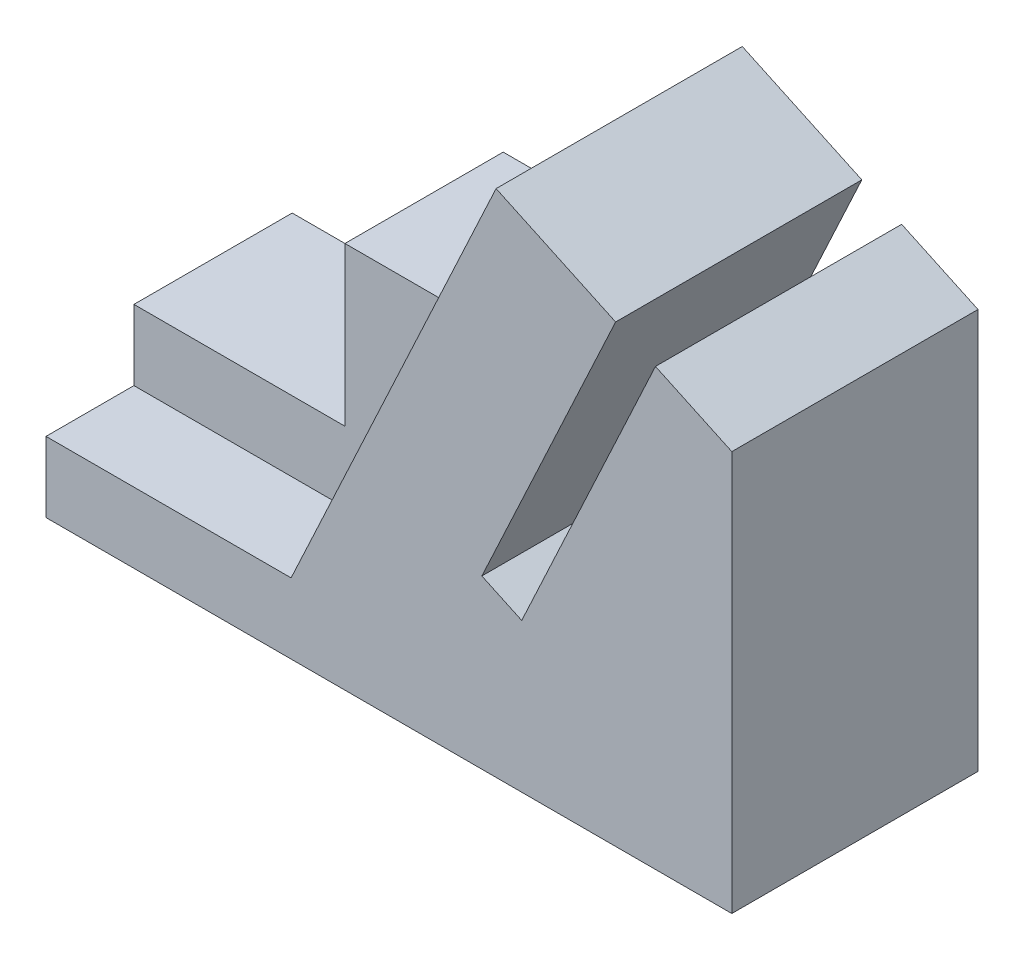
ISO-10303-21;
HEADER;
FILE_DESCRIPTION(('STEP AP214'),'2;1');
FILE_NAME('part.step','',(''),(''),'','','');
FILE_SCHEMA(('AUTOMOTIVE_DESIGN { 1 0 10303 214 1 1 1 1 }'));
ENDSEC;
DATA;
#1=APPLICATION_CONTEXT('core data for automotive mechanical design processes');
#2=APPLICATION_PROTOCOL_DEFINITION('international standard','automotive_design',2000,#1);
#3=PRODUCT_CONTEXT('',#1,'mechanical');
#4=PRODUCT('Part','Part','',(#3));
#5=PRODUCT_RELATED_PRODUCT_CATEGORY('part','',(#4));
#6=PRODUCT_DEFINITION_FORMATION('','',#4);
#7=PRODUCT_DEFINITION_CONTEXT('part definition',#1,'design');
#8=PRODUCT_DEFINITION('design','',#6,#7);
#9=PRODUCT_DEFINITION_SHAPE('','',#8);
#10=(LENGTH_UNIT() NAMED_UNIT(*) SI_UNIT(.MILLI.,.METRE.));
#11=(NAMED_UNIT(*) PLANE_ANGLE_UNIT() SI_UNIT($,.RADIAN.));
#12=(NAMED_UNIT(*) SI_UNIT($,.STERADIAN.) SOLID_ANGLE_UNIT());
#13=UNCERTAINTY_MEASURE_WITH_UNIT(LENGTH_MEASURE(1.E-05),#10,'distance_accuracy_value','');
#14=(GEOMETRIC_REPRESENTATION_CONTEXT(3) GLOBAL_UNCERTAINTY_ASSIGNED_CONTEXT((#13)) GLOBAL_UNIT_ASSIGNED_CONTEXT((#10,
#11,#12)) REPRESENTATION_CONTEXT('',''));
#15=CARTESIAN_POINT('',(0.,0.,0.));
#16=DIRECTION('',(0.,0.,1.));
#17=DIRECTION('',(1.,0.,0.));
#18=AXIS2_PLACEMENT_3D('',#15,#16,#17);
#19=CARTESIAN_POINT('',(0.,0.,3.99999999999999));
#20=DIRECTION('',(0.,0.,-1.));
#21=DIRECTION('',(-1.,0.,0.));
#22=AXIS2_PLACEMENT_3D('',#19,#20,#21);
#23=PLANE('',#22);
#24=DIRECTION('',(-0.422618261740697,-0.906307787036651,0.));
#25=VECTOR('',#24,1.);
#26=CARTESIAN_POINT('',(-12.2013617281793,5.68958841376926,3.99999999999999));
#27=LINE('',#26,#25);
#28=CARTESIAN_POINT('',(1.00000000000001,34.,3.99999999999999));
#29=VERTEX_POINT('',#28);
#30=CARTESIAN_POINT('',(-11.1239991120298,8.,3.99999999999999));
#31=VERTEX_POINT('',#30);
#32=EDGE_CURVE('E11',#29,#31,#27,.T.);
#33=ORIENTED_EDGE('',*,*,#32,.F.);
#34=DIRECTION('',(1.,0.,0.));
#35=VECTOR('',#34,1.);
#36=CARTESIAN_POINT('',(-15.,34.,3.99999999999999));
#37=LINE('',#36,#35);
#38=CARTESIAN_POINT('',(-15.,34.,3.99999999999999));
#39=VERTEX_POINT('',#38);
#40=EDGE_CURVE('E203',#39,#29,#37,.T.);
#41=ORIENTED_EDGE('',*,*,#40,.F.);
#42=DIRECTION('',(0.,1.,0.));
#43=VECTOR('',#42,1.);
#44=CARTESIAN_POINT('',(-15.,16.,3.99999999999999));
#45=LINE('',#44,#43);
#46=CARTESIAN_POINT('',(-15.,16.,3.99999999999999));
#47=VERTEX_POINT('',#46);
#48=EDGE_CURVE('E196',#47,#39,#45,.T.);
#49=ORIENTED_EDGE('',*,*,#48,.F.);
#50=DIRECTION('',(1.,0.,0.));
#51=VECTOR('',#50,1.);
#52=CARTESIAN_POINT('',(-39.,16.,3.99999999999999));
#53=LINE('',#52,#51);
#54=CARTESIAN_POINT('',(-39.,16.,3.99999999999999));
#55=VERTEX_POINT('',#54);
#56=EDGE_CURVE('E194',#55,#47,#53,.T.);
#57=ORIENTED_EDGE('',*,*,#56,.F.);
#58=DIRECTION('',(0.,1.,0.));
#59=VECTOR('',#58,1.);
#60=CARTESIAN_POINT('',(-39.,8.,3.99999999999999));
#61=LINE('',#60,#59);
#62=CARTESIAN_POINT('',(-39.,8.,3.99999999999999));
#63=VERTEX_POINT('',#62);
#64=EDGE_CURVE('E191',#63,#55,#61,.T.);
#65=ORIENTED_EDGE('',*,*,#64,.F.);
#66=DIRECTION('',(-1.,0.,0.));
#67=VECTOR('',#66,1.);
#68=CARTESIAN_POINT('',(1.00000000000001,8.,3.99999999999999));
#69=LINE('',#68,#67);
#70=EDGE_CURVE('E56',#31,#63,#69,.T.);
#71=ORIENTED_EDGE('',*,*,#70,.F.);
#72=EDGE_LOOP('',(#33,#41,#49,#57,#65,#71));
#73=FACE_BOUND('',#72,.T.);
#74=ADVANCED_FACE('F39',(#73),#23,.F.);
#75=CARTESIAN_POINT('',(39.,8.,-14.));
#76=DIRECTION('',(-1.,0.,0.));
#77=DIRECTION('',(0.,0.,1.));
#78=AXIS2_PLACEMENT_3D('',#75,#76,#77);
#79=PLANE('',#78);
#80=DIRECTION('',(0.,0.,-1.));
#81=VECTOR('',#80,1.);
#82=CARTESIAN_POINT('',(39.,0.,-14.));
#83=LINE('',#82,#81);
#84=CARTESIAN_POINT('',(39.,0.,14.));
#85=VERTEX_POINT('',#84);
#86=CARTESIAN_POINT('',(39.,0.,-14.));
#87=VERTEX_POINT('',#86);
#88=EDGE_CURVE('E214',#85,#87,#83,.T.);
#89=ORIENTED_EDGE('',*,*,#88,.T.);
#90=DIRECTION('',(0.,-1.,0.));
#91=VECTOR('',#90,1.);
#92=CARTESIAN_POINT('',(39.,8.,-14.));
#93=LINE('',#92,#91);
#94=CARTESIAN_POINT('',(39.,45.4989369594061,-14.));
#95=VERTEX_POINT('',#94);
#96=EDGE_CURVE('E50',#95,#87,#93,.T.);
#97=ORIENTED_EDGE('',*,*,#96,.F.);
#98=DIRECTION('',(0.,0.,1.));
#99=VECTOR('',#98,1.);
#100=CARTESIAN_POINT('',(39.,45.4989369594061,-84.7984130258777));
#101=LINE('',#100,#99);
#102=CARTESIAN_POINT('',(39.,45.4989369594061,14.));
#103=VERTEX_POINT('',#102);
#104=EDGE_CURVE('E179',#95,#103,#101,.T.);
#105=ORIENTED_EDGE('',*,*,#104,.T.);
#106=DIRECTION('',(0.,-1.,0.));
#107=VECTOR('',#106,1.);
#108=CARTESIAN_POINT('',(39.,8.,14.));
#109=LINE('',#108,#107);
#110=EDGE_CURVE('E229',#103,#85,#109,.T.);
#111=ORIENTED_EDGE('',*,*,#110,.T.);
#112=EDGE_LOOP('',(#89,#97,#105,#111));
#113=FACE_BOUND('',#112,.T.);
#114=ADVANCED_FACE('F41',(#113),#79,.F.);
#115=CARTESIAN_POINT('',(-39.,8.,-14.));
#116=DIRECTION('',(0.,0.,1.));
#117=DIRECTION('',(1.,0.,0.));
#118=AXIS2_PLACEMENT_3D('',#115,#116,#117);
#119=PLANE('',#118);
#120=DIRECTION('',(1.,0.,0.));
#121=VECTOR('',#120,1.);
#122=CARTESIAN_POINT('',(-15.,34.,-14.));
#123=LINE('',#122,#121);
#124=CARTESIAN_POINT('',(-15.,34.,-14.));
#125=VERTEX_POINT('',#124);
#126=CARTESIAN_POINT('',(1.00000000000001,34.,-14.));
#127=VERTEX_POINT('',#126);
#128=EDGE_CURVE('E195',#125,#127,#123,.T.);
#129=ORIENTED_EDGE('',*,*,#128,.T.);
#130=DIRECTION('',(-0.422618261740697,-0.906307787036651,0.));
#131=VECTOR('',#130,1.);
#132=CARTESIAN_POINT('',(-11.1239991120298,8.,-14.));
#133=LINE('',#132,#131);
#134=CARTESIAN_POINT('',(12.1913837957199,58.,-14.));
#135=VERTEX_POINT('',#134);
#136=EDGE_CURVE('E167',#135,#127,#133,.T.);
#137=ORIENTED_EDGE('',*,*,#136,.F.);
#138=DIRECTION('',(-0.906307787036651,0.422618261740696,0.));
#139=VECTOR('',#138,1.);
#140=CARTESIAN_POINT('',(12.1913837957199,58.,-14.));
#141=LINE('',#140,#139);
#142=CARTESIAN_POINT('',(25.7860006012697,51.6607260738895,-14.));
#143=VERTEX_POINT('',#142);
#144=EDGE_CURVE('E148',#143,#135,#141,.T.);
#145=ORIENTED_EDGE('',*,*,#144,.F.);
#146=DIRECTION('',(0.422618261740697,0.906307787036651,0.));
#147=VECTOR('',#146,1.);
#148=CARTESIAN_POINT('',(25.7860006012697,51.6607260738895,-14.));
#149=LINE('',#148,#147);
#150=CARTESIAN_POINT('',(10.5717431786046,19.0336457405701,-14.));
#151=VERTEX_POINT('',#150);
#152=EDGE_CURVE('E273',#151,#143,#149,.T.);
#153=ORIENTED_EDGE('',*,*,#152,.F.);
#154=DIRECTION('',(-0.906307787036651,0.422618261740696,0.));
#155=VECTOR('',#154,1.);
#156=CARTESIAN_POINT('',(10.5717431786046,19.0336457405701,-14.));
#157=LINE('',#156,#155);
#158=CARTESIAN_POINT('',(15.1032821137878,16.9205544318666,-14.));
#159=VERTEX_POINT('',#158);
#160=EDGE_CURVE('E269',#159,#151,#157,.T.);
#161=ORIENTED_EDGE('',*,*,#160,.F.);
#162=DIRECTION('',(-0.422618261740696,-0.906307787036652,0.));
#163=VECTOR('',#162,1.);
#164=CARTESIAN_POINT('',(15.1032821137878,16.9205544318666,-14.));
#165=LINE('',#164,#163);
#166=CARTESIAN_POINT('',(30.3175395364529,49.5476347651861,-14.));
#167=VERTEX_POINT('',#166);
#168=EDGE_CURVE('E277',#167,#159,#165,.T.);
#169=ORIENTED_EDGE('',*,*,#168,.F.);
#170=DIRECTION('',(-0.906307787036652,0.422618261740696,0.));
#171=VECTOR('',#170,1.);
#172=CARTESIAN_POINT('',(30.3175395364529,49.5476347651861,-14.));
#173=LINE('',#172,#171);
#174=EDGE_CURVE('E147',#95,#167,#173,.T.);
#175=ORIENTED_EDGE('',*,*,#174,.F.);
#176=ORIENTED_EDGE('',*,*,#96,.T.);
#177=DIRECTION('',(-1.,0.,0.));
#178=VECTOR('',#177,1.);
#179=CARTESIAN_POINT('',(-39.,0.,-14.));
#180=LINE('',#179,#178);
#181=CARTESIAN_POINT('',(-39.,0.,-14.));
#182=VERTEX_POINT('',#181);
#183=EDGE_CURVE('E228',#87,#182,#180,.T.);
#184=ORIENTED_EDGE('',*,*,#183,.T.);
#185=DIRECTION('',(0.,-1.,0.));
#186=VECTOR('',#185,1.);
#187=CARTESIAN_POINT('',(-39.,8.,-14.));
#188=LINE('',#187,#186);
#189=CARTESIAN_POINT('',(-39.,16.,-14.));
#190=VERTEX_POINT('',#189);
#191=EDGE_CURVE('E239',#190,#182,#188,.T.);
#192=ORIENTED_EDGE('',*,*,#191,.F.);
#193=DIRECTION('',(1.,0.,0.));
#194=VECTOR('',#193,1.);
#195=CARTESIAN_POINT('',(-39.,16.,-14.));
#196=LINE('',#195,#194);
#197=CARTESIAN_POINT('',(-15.,16.,-14.));
#198=VERTEX_POINT('',#197);
#199=EDGE_CURVE('E202',#190,#198,#196,.T.);
#200=ORIENTED_EDGE('',*,*,#199,.T.);
#201=DIRECTION('',(0.,1.,0.));
#202=VECTOR('',#201,1.);
#203=CARTESIAN_POINT('',(-15.,16.,-14.));
#204=LINE('',#203,#202);
#205=EDGE_CURVE('E208',#198,#125,#204,.T.);
#206=ORIENTED_EDGE('',*,*,#205,.T.);
#207=EDGE_LOOP('',(#129,#137,#145,#153,#161,#169,#175,#176,#184,#192,#200,#206));
#208=FACE_BOUND('',#207,.T.);
#209=ADVANCED_FACE('F243',(#208),#119,.F.);
#210=CARTESIAN_POINT('',(-39.,8.,-14.));
#211=DIRECTION('',(1.,0.,0.));
#212=DIRECTION('',(0.,0.,-1.));
#213=AXIS2_PLACEMENT_3D('',#210,#211,#212);
#214=PLANE('',#213);
#215=DIRECTION('',(0.,0.,1.));
#216=VECTOR('',#215,1.);
#217=CARTESIAN_POINT('',(-39.,0.,-14.));
#218=LINE('',#217,#216);
#219=CARTESIAN_POINT('',(-39.,0.,14.));
#220=VERTEX_POINT('',#219);
#221=EDGE_CURVE('E231',#182,#220,#218,.T.);
#222=ORIENTED_EDGE('',*,*,#221,.T.);
#223=DIRECTION('',(0.,-1.,0.));
#224=VECTOR('',#223,1.);
#225=CARTESIAN_POINT('',(-39.,8.,14.));
#226=LINE('',#225,#224);
#227=CARTESIAN_POINT('',(-39.,8.,14.));
#228=VERTEX_POINT('',#227);
#229=EDGE_CURVE('E237',#228,#220,#226,.T.);
#230=ORIENTED_EDGE('',*,*,#229,.F.);
#231=DIRECTION('',(0.,0.,1.));
#232=VECTOR('',#231,1.);
#233=CARTESIAN_POINT('',(-39.,8.,-14.));
#234=LINE('',#233,#232);
#235=EDGE_CURVE('E225',#63,#228,#234,.T.);
#236=ORIENTED_EDGE('',*,*,#235,.F.);
#237=ORIENTED_EDGE('',*,*,#64,.T.);
#238=DIRECTION('',(0.,0.,-1.));
#239=VECTOR('',#238,1.);
#240=CARTESIAN_POINT('',(-39.,16.,3.99999999999999));
#241=LINE('',#240,#239);
#242=EDGE_CURVE('E204',#55,#190,#241,.T.);
#243=ORIENTED_EDGE('',*,*,#242,.T.);
#244=ORIENTED_EDGE('',*,*,#191,.T.);
#245=EDGE_LOOP('',(#222,#230,#236,#237,#243,#244));
#246=FACE_BOUND('',#245,.T.);
#247=ADVANCED_FACE('F254',(#246),#214,.F.);
#248=CARTESIAN_POINT('',(-39.,8.,14.));
#249=DIRECTION('',(0.,0.,-1.));
#250=DIRECTION('',(-1.,0.,0.));
#251=AXIS2_PLACEMENT_3D('',#248,#249,#250);
#252=PLANE('',#251);
#253=DIRECTION('',(1.,0.,0.));
#254=VECTOR('',#253,1.);
#255=CARTESIAN_POINT('',(-39.,0.,14.));
#256=LINE('',#255,#254);
#257=EDGE_CURVE('E221',#220,#85,#256,.T.);
#258=ORIENTED_EDGE('',*,*,#257,.T.);
#259=ORIENTED_EDGE('',*,*,#110,.F.);
#260=DIRECTION('',(0.906307787036651,-0.422618261740696,0.));
#261=VECTOR('',#260,1.);
#262=CARTESIAN_POINT('',(30.3175395364529,49.5476347651861,14.));
#263=LINE('',#262,#261);
#264=CARTESIAN_POINT('',(30.3175395364529,49.5476347651861,14.));
#265=VERTEX_POINT('',#264);
#266=EDGE_CURVE('E176',#265,#103,#263,.T.);
#267=ORIENTED_EDGE('',*,*,#266,.F.);
#268=DIRECTION('',(0.422618261740696,0.906307787036651,0.));
#269=VECTOR('',#268,1.);
#270=CARTESIAN_POINT('',(15.1032821137878,16.9205544318666,14.));
#271=LINE('',#270,#269);
#272=CARTESIAN_POINT('',(15.1032821137878,16.9205544318666,14.));
#273=VERTEX_POINT('',#272);
#274=EDGE_CURVE('E175',#273,#265,#271,.T.);
#275=ORIENTED_EDGE('',*,*,#274,.F.);
#276=DIRECTION('',(0.906307787036652,-0.422618261740696,0.));
#277=VECTOR('',#276,1.);
#278=CARTESIAN_POINT('',(10.5717431786046,19.0336457405701,14.));
#279=LINE('',#278,#277);
#280=CARTESIAN_POINT('',(10.5717431786046,19.0336457405701,14.));
#281=VERTEX_POINT('',#280);
#282=EDGE_CURVE('E168',#281,#273,#279,.T.);
#283=ORIENTED_EDGE('',*,*,#282,.F.);
#284=DIRECTION('',(-0.422618261740696,-0.906307787036651,0.));
#285=VECTOR('',#284,1.);
#286=CARTESIAN_POINT('',(25.7860006012697,51.6607260738895,14.));
#287=LINE('',#286,#285);
#288=CARTESIAN_POINT('',(25.7860006012697,51.6607260738895,14.));
#289=VERTEX_POINT('',#288);
#290=EDGE_CURVE('E157',#289,#281,#287,.T.);
#291=ORIENTED_EDGE('',*,*,#290,.F.);
#292=DIRECTION('',(0.906307787036651,-0.422618261740696,0.));
#293=VECTOR('',#292,1.);
#294=CARTESIAN_POINT('',(12.1913837957199,58.,14.));
#295=LINE('',#294,#293);
#296=CARTESIAN_POINT('',(12.1913837957199,58.,14.));
#297=VERTEX_POINT('',#296);
#298=EDGE_CURVE('E145',#297,#289,#295,.T.);
#299=ORIENTED_EDGE('',*,*,#298,.F.);
#300=DIRECTION('',(0.422618261740697,0.906307787036651,0.));
#301=VECTOR('',#300,1.);
#302=CARTESIAN_POINT('',(-11.1239991120298,8.,14.));
#303=LINE('',#302,#301);
#304=CARTESIAN_POINT('',(-11.1239991120298,8.,14.));
#305=VERTEX_POINT('',#304);
#306=EDGE_CURVE('E156',#305,#297,#303,.T.);
#307=ORIENTED_EDGE('',*,*,#306,.F.);
#308=DIRECTION('',(1.,0.,0.));
#309=VECTOR('',#308,1.);
#310=CARTESIAN_POINT('',(-39.,8.,14.));
#311=LINE('',#310,#309);
#312=EDGE_CURVE('E53',#228,#305,#311,.T.);
#313=ORIENTED_EDGE('',*,*,#312,.F.);
#314=ORIENTED_EDGE('',*,*,#229,.T.);
#315=EDGE_LOOP('',(#258,#259,#267,#275,#283,#291,#299,#307,#313,#314));
#316=FACE_BOUND('',#315,.T.);
#317=ADVANCED_FACE('F154',(#316),#252,.F.);
#318=CARTESIAN_POINT('',(0.,8.,0.));
#319=DIRECTION('',(0.,1.,0.));
#320=DIRECTION('',(0.,0.,1.));
#321=AXIS2_PLACEMENT_3D('',#318,#319,#320);
#322=PLANE('',#321);
#323=DIRECTION('',(0.,0.,1.));
#324=VECTOR('',#323,1.);
#325=CARTESIAN_POINT('',(-11.1239991120298,8.,-84.7984130258777));
#326=LINE('',#325,#324);
#327=EDGE_CURVE('E162',#31,#305,#326,.T.);
#328=ORIENTED_EDGE('',*,*,#327,.F.);
#329=ORIENTED_EDGE('',*,*,#70,.T.);
#330=ORIENTED_EDGE('',*,*,#235,.T.);
#331=ORIENTED_EDGE('',*,*,#312,.T.);
#332=EDGE_LOOP('',(#328,#329,#330,#331));
#333=FACE_BOUND('',#332,.T.);
#334=ADVANCED_FACE('F291',(#333),#322,.T.);
#335=CARTESIAN_POINT('',(0.,0.,0.));
#336=DIRECTION('',(0.,1.,0.));
#337=DIRECTION('',(0.,0.,1.));
#338=AXIS2_PLACEMENT_3D('',#335,#336,#337);
#339=PLANE('',#338);
#340=ORIENTED_EDGE('',*,*,#88,.F.);
#341=ORIENTED_EDGE('',*,*,#257,.F.);
#342=ORIENTED_EDGE('',*,*,#221,.F.);
#343=ORIENTED_EDGE('',*,*,#183,.F.);
#344=EDGE_LOOP('',(#340,#341,#342,#343));
#345=FACE_BOUND('',#344,.T.);
#346=ADVANCED_FACE('F253',(#345),#339,.F.);
#347=CARTESIAN_POINT('',(-15.,34.,3.99999999999999));
#348=DIRECTION('',(0.,1.,0.));
#349=DIRECTION('',(0.,0.,1.));
#350=AXIS2_PLACEMENT_3D('',#347,#348,#349);
#351=PLANE('',#350);
#352=ORIENTED_EDGE('',*,*,#128,.F.);
#353=DIRECTION('',(0.,0.,-1.));
#354=VECTOR('',#353,1.);
#355=CARTESIAN_POINT('',(-15.,34.,3.99999999999999));
#356=LINE('',#355,#354);
#357=EDGE_CURVE('E216',#39,#125,#356,.T.);
#358=ORIENTED_EDGE('',*,*,#357,.F.);
#359=ORIENTED_EDGE('',*,*,#40,.T.);
#360=DIRECTION('',(0.,0.,-1.));
#361=VECTOR('',#360,1.);
#362=CARTESIAN_POINT('',(1.00000000000001,34.,3.99999999999999));
#363=LINE('',#362,#361);
#364=EDGE_CURVE('E213',#29,#127,#363,.T.);
#365=ORIENTED_EDGE('',*,*,#364,.T.);
#366=EDGE_LOOP('',(#352,#358,#359,#365));
#367=FACE_BOUND('',#366,.T.);
#368=ADVANCED_FACE('F285',(#367),#351,.T.);
#369=CARTESIAN_POINT('',(-15.,16.,3.99999999999999));
#370=DIRECTION('',(-1.,0.,0.));
#371=DIRECTION('',(0.,-1.,0.));
#372=AXIS2_PLACEMENT_3D('',#369,#370,#371);
#373=PLANE('',#372);
#374=ORIENTED_EDGE('',*,*,#205,.F.);
#375=DIRECTION('',(0.,0.,-1.));
#376=VECTOR('',#375,1.);
#377=CARTESIAN_POINT('',(-15.,16.,3.99999999999999));
#378=LINE('',#377,#376);
#379=EDGE_CURVE('E217',#47,#198,#378,.T.);
#380=ORIENTED_EDGE('',*,*,#379,.F.);
#381=ORIENTED_EDGE('',*,*,#48,.T.);
#382=ORIENTED_EDGE('',*,*,#357,.T.);
#383=EDGE_LOOP('',(#374,#380,#381,#382));
#384=FACE_BOUND('',#383,.T.);
#385=ADVANCED_FACE('F288',(#384),#373,.T.);
#386=CARTESIAN_POINT('',(-39.,16.,3.99999999999999));
#387=DIRECTION('',(0.,1.,0.));
#388=DIRECTION('',(-1.,0.,0.));
#389=AXIS2_PLACEMENT_3D('',#386,#387,#388);
#390=PLANE('',#389);
#391=ORIENTED_EDGE('',*,*,#199,.F.);
#392=ORIENTED_EDGE('',*,*,#242,.F.);
#393=ORIENTED_EDGE('',*,*,#56,.T.);
#394=ORIENTED_EDGE('',*,*,#379,.T.);
#395=EDGE_LOOP('',(#391,#392,#393,#394));
#396=FACE_BOUND('',#395,.T.);
#397=ADVANCED_FACE('F295',(#396),#390,.T.);
#398=CARTESIAN_POINT('',(-11.1239991120298,8.,-84.7984130258777));
#399=DIRECTION('',(0.906307787036651,-0.422618261740697,0.));
#400=DIRECTION('',(0.422618261740697,0.906307787036651,0.));
#401=AXIS2_PLACEMENT_3D('',#398,#399,#400);
#402=PLANE('',#401);
#403=ORIENTED_EDGE('',*,*,#364,.F.);
#404=ORIENTED_EDGE('',*,*,#32,.T.);
#405=ORIENTED_EDGE('',*,*,#327,.T.);
#406=ORIENTED_EDGE('',*,*,#306,.T.);
#407=DIRECTION('',(0.,0.,1.));
#408=VECTOR('',#407,1.);
#409=CARTESIAN_POINT('',(12.1913837957199,58.,-84.7984130258777));
#410=LINE('',#409,#408);
#411=EDGE_CURVE('E139',#135,#297,#410,.T.);
#412=ORIENTED_EDGE('',*,*,#411,.F.);
#413=ORIENTED_EDGE('',*,*,#136,.T.);
#414=EDGE_LOOP('',(#403,#404,#405,#406,#412,#413));
#415=FACE_BOUND('',#414,.T.);
#416=ADVANCED_FACE('F165',(#415),#402,.F.);
#417=CARTESIAN_POINT('',(12.1913837957199,58.,-84.7984130258777));
#418=DIRECTION('',(-0.422618261740696,-0.906307787036652,0.));
#419=DIRECTION('',(0.906307787036651,-0.422618261740696,0.));
#420=AXIS2_PLACEMENT_3D('',#417,#418,#419);
#421=PLANE('',#420);
#422=DIRECTION('',(0.,0.,1.));
#423=VECTOR('',#422,1.);
#424=CARTESIAN_POINT('',(25.7860006012697,51.6607260738895,-84.7984130258777));
#425=LINE('',#424,#423);
#426=EDGE_CURVE('E151',#143,#289,#425,.T.);
#427=ORIENTED_EDGE('',*,*,#426,.F.);
#428=ORIENTED_EDGE('',*,*,#144,.T.);
#429=ORIENTED_EDGE('',*,*,#411,.T.);
#430=ORIENTED_EDGE('',*,*,#298,.T.);
#431=EDGE_LOOP('',(#427,#428,#429,#430));
#432=FACE_BOUND('',#431,.T.);
#433=ADVANCED_FACE('F141',(#432),#421,.F.);
#434=CARTESIAN_POINT('',(25.7860006012697,51.6607260738895,-84.7984130258777));
#435=DIRECTION('',(-0.906307787036651,0.422618261740697,0.));
#436=DIRECTION('',(-0.422618261740697,-0.906307787036651,0.));
#437=AXIS2_PLACEMENT_3D('',#434,#435,#436);
#438=PLANE('',#437);
#439=DIRECTION('',(0.,0.,1.));
#440=VECTOR('',#439,1.);
#441=CARTESIAN_POINT('',(10.5717431786046,19.0336457405701,-84.7984130258777));
#442=LINE('',#441,#440);
#443=EDGE_CURVE('E186',#151,#281,#442,.T.);
#444=ORIENTED_EDGE('',*,*,#443,.F.);
#445=ORIENTED_EDGE('',*,*,#152,.T.);
#446=ORIENTED_EDGE('',*,*,#426,.T.);
#447=ORIENTED_EDGE('',*,*,#290,.T.);
#448=EDGE_LOOP('',(#444,#445,#446,#447));
#449=FACE_BOUND('',#448,.T.);
#450=ADVANCED_FACE('F272',(#449),#438,.F.);
#451=CARTESIAN_POINT('',(10.5717431786046,19.0336457405701,-84.7984130258777));
#452=DIRECTION('',(-0.422618261740696,-0.906307787036651,0.));
#453=DIRECTION('',(0.906307787036651,-0.422618261740696,0.));
#454=AXIS2_PLACEMENT_3D('',#451,#452,#453);
#455=PLANE('',#454);
#456=DIRECTION('',(0.,0.,1.));
#457=VECTOR('',#456,1.);
#458=CARTESIAN_POINT('',(15.1032821137878,16.9205544318666,-84.7984130258777));
#459=LINE('',#458,#457);
#460=EDGE_CURVE('E183',#159,#273,#459,.T.);
#461=ORIENTED_EDGE('',*,*,#460,.F.);
#462=ORIENTED_EDGE('',*,*,#160,.T.);
#463=ORIENTED_EDGE('',*,*,#443,.T.);
#464=ORIENTED_EDGE('',*,*,#282,.T.);
#465=EDGE_LOOP('',(#461,#462,#463,#464));
#466=FACE_BOUND('',#465,.T.);
#467=ADVANCED_FACE('F270',(#466),#455,.F.);
#468=CARTESIAN_POINT('',(15.1032821137878,16.9205544318666,-84.7984130258777));
#469=DIRECTION('',(0.906307787036652,-0.422618261740696,0.));
#470=DIRECTION('',(0.422618261740696,0.906307787036652,0.));
#471=AXIS2_PLACEMENT_3D('',#468,#469,#470);
#472=PLANE('',#471);
#473=DIRECTION('',(0.,0.,1.));
#474=VECTOR('',#473,1.);
#475=CARTESIAN_POINT('',(30.3175395364529,49.5476347651861,-84.7984130258777));
#476=LINE('',#475,#474);
#477=EDGE_CURVE('E181',#167,#265,#476,.T.);
#478=ORIENTED_EDGE('',*,*,#477,.F.);
#479=ORIENTED_EDGE('',*,*,#168,.T.);
#480=ORIENTED_EDGE('',*,*,#460,.T.);
#481=ORIENTED_EDGE('',*,*,#274,.T.);
#482=EDGE_LOOP('',(#478,#479,#480,#481));
#483=FACE_BOUND('',#482,.T.);
#484=ADVANCED_FACE('F262',(#483),#472,.F.);
#485=CARTESIAN_POINT('',(30.3175395364529,49.5476347651861,-84.7984130258777));
#486=DIRECTION('',(-0.422618261740696,-0.906307787036652,0.));
#487=DIRECTION('',(0.906307787036652,-0.422618261740696,0.));
#488=AXIS2_PLACEMENT_3D('',#485,#486,#487);
#489=PLANE('',#488);
#490=ORIENTED_EDGE('',*,*,#104,.F.);
#491=ORIENTED_EDGE('',*,*,#174,.T.);
#492=ORIENTED_EDGE('',*,*,#477,.T.);
#493=ORIENTED_EDGE('',*,*,#266,.T.);
#494=EDGE_LOOP('',(#490,#491,#492,#493));
#495=FACE_BOUND('',#494,.T.);
#496=ADVANCED_FACE('F257',(#495),#489,.F.);
#497=CLOSED_SHELL('',(#74,#114,#209,#247,#317,#334,#346,#368,#385,#397,#416,#433,#450,#467,#484,#496));
#498=MANIFOLD_SOLID_BREP('B2',#497);
#499=ADVANCED_BREP_SHAPE_REPRESENTATION('',(#18,#498),#14);
#500=SHAPE_DEFINITION_REPRESENTATION(#9,#499);
ENDSEC;
END-ISO-10303-21;
